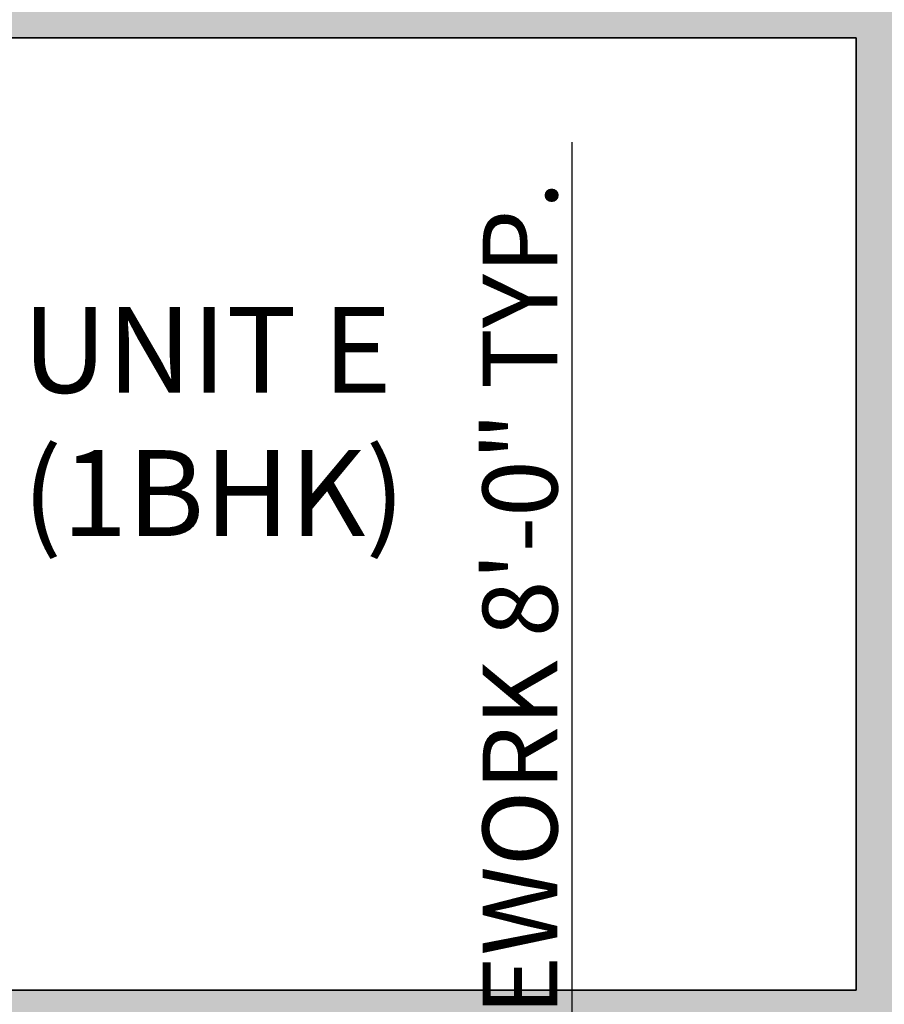
# Model space of a CAD drawing. Units: inches. Extents: x 2083 to 3317, y 1141 to 2115.
# Tile 89 of 256: x 2462 to 2600, y 1419 to 1577. Entities that reach past the tile are written whole.
import ezdxf

# ---------------------------------------------------------------- set-up
doc = ezdxf.new("R2010")
doc.units = ezdxf.units.IN
for name, color, linetype, lineweight in [('A-ANNO-DIMS', 2, 'Continuous', 18), ('A-AREA-IDEN', 7, 'Continuous', 25), ('A-WALL', 7, 'Continuous', 35)]:
    doc.layers.add(name, color=color, linetype=linetype, lineweight=lineweight)
doc.layers.add('A-WALL-PATT', color=251, linetype='Continuous', lineweight=13, true_color=0x636466)
doc.styles.get("Standard").update_dxf_attribs({"font": 'arial.ttf'})
doc.dimstyles.new('ISO-25', dxfattribs={"dimtxt": 12, "dimasz": 12, "dimexe": 1.25, "dimexo": 0.625, "dimtad": 1, "dimlunit": 3, "dimtxsty": 'Standard', "dimcen": 2.5, "dimadec": 0, "dimazin": 0, "dimtfac": 1, "dimtmove": 0, "dimatfit": 3, "dimfxl": 1, "dimarcsym": 0})

# ---------------------------------------------------------------- blocks, each defined once
blk = doc.blocks.new('*D24')
at = {"layer": 'A-ANNO-DIMS', "color": 0, "lineweight": -2, "transparency": 16777216}
for p, q in [((2550.36, 1368.26), (2550.36, 1556.98)), ((2536.58, 1368.26), (2551.61, 1368.26)), ((2550.36, 1284.26), (2550.36, 1356.26)), ((2536.58, 1272.26), (2551.61, 1272.26))]:
    blk.add_line(p, q, dxfattribs=at)
at = {"layer": 'A-ANNO-DIMS', "color": 0, "transparency": 16777216}
for points in [[(2548.36, 1356.26), (2552.36, 1356.26), (2550.36, 1368.26)], [(2548.36, 1284.26), (2552.36, 1284.26), (2550.36, 1272.26)]]:
    blk.add_solid(points, dxfattribs=at)
at = {"layer": 'Defpoints', "color": 0, "transparency": 16777216}
for p in [(2535.96, 1368.26), (2550.36, 1368.26), (2535.96, 1272.26)]:
    blk.add_point(p, dxfattribs=at)
at = {"layer": 'A-ANNO-DIMS', "color": 0, "transparency": 16777216, "insert": (2543.53, 1468.62), "char_height": 12, "attachment_point": 5, "rotation": 90}
blk.add_mtext('CASEWORK 8\'-0" TYP.', dxfattribs=at)

msp = doc.modelspace()

# ---------------------------------------------------------------- hatches: boundary and pattern name
at = {"layer": 'A-WALL-PATT'}
h = msp.add_hatch(color=256, dxfattribs=at)
h.dxf.hatch_style = 1
h.paths.add_polyline_path([(3126.96, 2020.761), (2748.96, 2020.761), (2604.96, 2020.761), (2226.96, 2020.761), (2226.96, 1702.761), (2466.96, 1702.761), (2466.96, 1582.761), (2418.96, 1582.761), (2418.96, 1477.761), (2226.96, 1477.761), (2226.96, 1263.261), (2544.96, 1263.261), (2544.96, 1411.761), (2604.96, 1411.761), (2685.96, 1411.761), (2685.96, 1420.761), (2604.96, 1420.761), (2604.96, 1573.761), (2604.96, 1702.761), (2604.96, 2011.761), (2748.96, 2011.761), (2748.96, 1702.761), (2862.96, 1702.761), (2862.96, 1621.761), (2871.96, 1621.761), (2871.96, 1702.761), (2883.96, 1702.761), (2883.96, 1706.939, -0.0264593), (2883.96, 1711.761), (2757.96, 1711.761), (2757.96, 1807.761), (2787.96, 1807.761), (2787.96, 1812.261), (2757.96, 1812.261), (2757.96, 2011.761), (2877.96, 2011.761), (2877.96, 1812.261), (2847.96, 1812.261), (2847.96, 1807.761), (2889.836, 1807.761), (2889.836, 1812.261), (2882.46, 1812.261), (2882.46, 2011.761), (3117.96, 2011.761), (3117.96, 1812.261), (2937.836, 1812.261), (2937.836, 1807.761), (2995.71, 1807.761), (2995.71, 1796.118), (3000.21, 1796.118), (3000.21, 1807.761), (3117.96, 1807.761), (3117.96, 1711.761), (3000.21, 1711.761), (3000.21, 1760.118), (2998.573, 1760.118, -0.020711), (2995.71, 1760.118), (2995.71, 1711.761), (2931.96, 1711.761), (2931.96, 1702.761), (3126.96, 1702.761)])
h.paths.add_polyline_path([(2471.46, 2011.761), (2471.46, 1810.011), (2462.717, 1810.011), (2462.717, 1805.511), (2505.96, 1805.511), (2505.96, 1810.011), (2475.96, 1810.011), (2475.96, 2011.761), (2595.96, 2011.761), (2595.96, 1810.011), (2565.96, 1810.011), (2565.96, 1805.511), (2595.96, 1805.511), (2595.96, 1711.761), (2235.96, 1711.761), (2235.96, 1805.511), (2353.71, 1805.511), (2353.71, 1796.054), (2358.21, 1796.054), (2358.21, 1805.511), (2414.717, 1805.511), (2414.717, 1810.011), (2235.96, 1810.011), (2235.96, 2011.761)], flags=16)
h.paths.add_polyline_path([(2270.205, 1994.61), (2270.205, 1970.61), (2246.205, 1970.61), (2246.205, 1994.61)], flags=0)
edge = h.paths.add_edge_path(flags=0)
edge.add_ellipse((2332.027, 1899.798), major_axis=(-3.043, 3.043), ratio=0.1682525, start_angle=-161.33217, end_angle=-156.30711, ccw=False)
edge.add_ellipse((2333.082, 1898.744), major_axis=(-1.055, 1.055), ratio=0.4535321, start_angle=-123.37102, end_angle=-94.15911)
edge = h.paths.add_edge_path(flags=0)
edge.add_ellipse((2332.027, 1968.876), major_axis=(3.043, 3.043), ratio=0.1682525, start_angle=18.66783, end_angle=23.69289)
edge.add_spline(control_points=[(2332.926, 1970.691), (2332.227, 1970.336), (2330.894, 1969.659), (2328.413, 1970.932), (2327.204, 1967.749), (2324.71, 1969.956), (2322.533, 1967.012), (2320.013, 1971.296), (2317.68, 1968.158), (2316.041, 1967.102), (2315.427, 1966.81)], knot_values=[0, 0, 0, 0, 2.2670587, 4.3245589, 6.6855835, 8.8786411, 11.121502, 14.300359, 17.7552837, 19.732645, 19.732645, 19.732645, 19.732645], degree=3, periodic=0)
edge.add_ellipse((2332.027, 1968.876), major_axis=(3.043, 3.043), ratio=0.1682525, start_angle=18.66783, end_angle=23.69289, ccw=False)
edge.add_ellipse((2333.082, 1969.931), major_axis=(1.055, 1.055), ratio=0.4535321, start_angle=56.62898, end_angle=85.84089, ccw=False)
edge = h.paths.add_edge_path(flags=0)
edge.add_spline(control_points=[(2296.428, 1967.988), (2293.628, 1965.336), (2287.704, 1959.727), (2299.744, 1949.996), (2294.533, 1935.669), (2290.573, 1920.604), (2293.394, 1909.974), (2296.185, 1904.967)], knot_values=[0.0991853, 0.0991853, 0.0991853, 0.0991853, 0.3453009, 0.6198217, 0.9826526, 1.3860932, 1.8105546, 1.8105546, 1.8105546, 1.8105546], degree=3, periodic=0)
edge.add_spline(control_points=[(2296.185, 1904.967), (2297.384, 1902.619), (2298.001, 1901.949), (2298.553, 1901.468)], knot_values=[0.0062457, 0.0062457, 0.0062457, 0.0062457, 0.0554759, 0.0554759, 0.0554759, 0.0554759], degree=3, periodic=0)
edge.add_spline(control_points=[(2298.553, 1901.468), (2297.259, 1900.923), (2295.225, 1900.232), (2293.06, 1900.614), (2292.101, 1900.788), (2292.09, 1900.791)], knot_values=[0.3128349, 0.3128349, 0.3128349, 0.3128349, 0.4017797, 0.4749867, 0.4759027, 0.4759027, 0.4759027, 0.4759027], degree=3, periodic=0)
edge.add_arc((2292.794, 1904.664), 3.937, 215.4209, 259.69818, ccw=False)
edge.add_spline(control_points=[(2289.585, 1902.382), (2289.477, 1902.535), (2289.368, 1902.688), (2289.261, 1902.841)], knot_values=[0.1028719, 0.1028719, 0.1028719, 0.1028719, 0.1168958, 0.1168958, 0.1168958, 0.1168958], degree=3, periodic=0)
edge.add_spline(control_points=[(2289.261, 1902.841), (2288.687, 1902.55), (2287.64, 1902.02), (2285.881, 1901.874), (2283.853, 1901.504), (2281.72, 1899.711), (2278.467, 1899.493), (2276.157, 1901.883), (2272.259, 1899.804), (2267.778, 1901.843), (2262.244, 1900.184), (2257.415, 1901.782), (2254.318, 1900.726), (2253.178, 1900.337)], knot_values=[0, 0, 0, 0, 1.9079767, 3.4771759, 5.261074, 7.9728515, 11.6802485, 13.7179214, 16.9395917, 22.789562, 27.5025027, 33.5952153, 37.1456181, 37.1456181, 37.1456181, 37.1456181], degree=3, periodic=0)
edge.add_line((2253.178, 1900.337), (2250.244, 1902.841))
edge.add_line((2250.244, 1902.841), (2250.244, 1965.833))
edge.add_line((2250.244, 1965.833), (2253.178, 1968.337))
edge.add_spline(control_points=[(2253.178, 1968.337), (2254.318, 1967.948), (2257.415, 1966.892), (2262.244, 1968.49), (2267.778, 1966.831), (2271.527, 1968.537), (2273.876, 1967.828), (2274.207, 1967.728)], knot_values=[0, 0, 0, 0, 0.0901802, 0.2449351, 0.3646438, 0.5132331, 0.5378548, 0.5378548, 0.5378548, 0.5378548], degree=3, periodic=0)
edge.add_arc((2274.353, 1963.793), 3.937, 72.05113, 92.12795, ccw=False)
edge.add_arc((2281.297, 1985.23), 18.596, 252.05113, 288.56572)
edge.add_arc((2292.317, 1956.029), 12.646, 71.02679, 113.77822, ccw=False)
edge = h.paths.add_edge_path(flags=0)
edge.add_spline(control_points=[(2274.899, 1951.856), (2275.066, 1951.617), (2275.233, 1951.377), (2275.398, 1951.136)], knot_values=[1.4099157, 1.4099157, 1.4099157, 1.4099157, 1.4315903, 1.4315903, 1.4315903, 1.4315903], degree=3, periodic=0)
edge.add_spline(control_points=[(2275.398, 1951.136), (2275.792, 1950.562), (2276.179, 1949.984), (2276.546, 1949.397)], knot_values=[1.3582378, 1.3582378, 1.3582378, 1.3582378, 1.4099157, 1.4099157, 1.4099157, 1.4099157], degree=3, periodic=0)
edge.add_line((2276.546, 1949.397), (2277.437, 1947.862))
edge.add_spline(control_points=[(2277.437, 1947.862), (2276.304, 1945.673), (2274.64, 1942.427), (2274.632, 1938.094), (2272.799, 1930.852), (2274.356, 1943.897), (2275.948, 1947.923), (2276.546, 1949.397)], knot_values=[0.0056315, 0.0056315, 0.0056315, 0.0056315, 0.1860139, 0.2660015, 0.3570872, 0.5963902, 0.7397317, 0.7397317, 0.7397317, 0.7397317], degree=3, periodic=0)
edge.add_spline(control_points=[(2276.546, 1949.397), (2276.179, 1949.984), (2275.792, 1950.562), (2275.398, 1951.136)], knot_values=[1.3582378, 1.3582378, 1.3582378, 1.3582378, 1.4099157, 1.4099157, 1.4099157, 1.4099157], degree=3, periodic=0)
edge.add_spline(control_points=[(2275.398, 1951.136), (2274.943, 1950.08), (2274.208, 1948.025), (2273.935, 1944.851), (2272.469, 1937.627), (2273.466, 1945.696), (2274.701, 1951.059), (2274.899, 1951.856)], knot_values=[0.1043639, 0.1043639, 0.1043639, 0.1043639, 0.1896363, 0.2696239, 0.3607096, 0.6000126, 0.6446217, 0.6446217, 0.6446217, 0.6446217], degree=3, periodic=0)
h.paths.add_polyline_path([(2269.168, 1963.128, -0.3575267), (2268.171, 1960.976, -0.0925607), (2268.171, 1939.436, -0.3575267), (2269.168, 1937.285, -0.3575267), (2267.016, 1938.282, -0.1647847), (2254.686, 1938.282, -0.3575267), (2252.534, 1937.285, -0.3575267), (2253.531, 1939.436, -0.0925607), (2253.531, 1960.976, -0.3575267), (2252.534, 1963.128, -0.3575267), (2254.686, 1962.131, -0.1647847), (2267.016, 1962.131, -0.3575267)], flags=0)
h.paths.add_polyline_path([(2248.874, 1967.802), (2248.874, 1957.028), (2249.458, 1957.028), (2249.458, 1911.647), (2248.874, 1911.647), (2248.874, 1900.873), (2246.512, 1900.873, 0.1973271), (2244.15, 1902.457), (2244.15, 1966.218, 0.1973271), (2246.512, 1967.802)], flags=0)
h.paths.add_polyline_path([(2269.168, 1931.389, -0.3575267), (2268.171, 1929.238, -0.0925607), (2268.171, 1907.698, -0.3575267), (2269.168, 1905.547, -0.3575267), (2267.016, 1906.544, -0.1647847), (2254.686, 1906.544, -0.3575267), (2252.534, 1905.547, -0.3575267), (2253.531, 1907.698, -0.0925607), (2253.531, 1929.238, -0.3575267), (2252.534, 1931.389, -0.3575267), (2254.686, 1930.392, -0.1647847), (2267.016, 1930.392, -0.3575267)], flags=0)
edge = h.paths.add_edge_path(flags=0)
edge.add_spline(control_points=[(2276.197, 1906.724), (2276.168, 1909.029), (2276.114, 1913.372), (2270.598, 1924.925), (2273.905, 1919.013), (2275.922, 1916.262), (2275.475, 1912.402), (2277.258, 1910.381), (2276.696, 1908.225), (2276.646, 1906.813), (2276.618, 1906.008)], knot_values=[0, 0, 0, 0, 8.6102597, 16.2212739, 18.8430575, 23.8048978, 27.4408283, 29.3561016, 31.2034776, 33.6506866, 33.6506866, 33.6506866, 33.6506866], degree=3, periodic=0)
edge.add_spline(control_points=[(2276.618, 1906.008), (2276.623, 1905.624), (2276.498, 1904.629), (2275.442, 1903.855), (2274.937, 1903.08), (2274.859, 1902.841)], knot_values=[0.1564884, 0.1564884, 0.1564884, 0.1564884, 0.1843975, 0.2313765, 0.2505985, 0.2505985, 0.2505985, 0.2505985], degree=3, periodic=0)
edge.add_line((2274.859, 1902.841), (2276.506, 1902.841))
edge.add_spline(control_points=[(2276.506, 1902.841), (2276.788, 1903.085), (2277.665, 1904.125), (2278.25, 1904.341), (2277.654, 1908.527), (2278.156, 1906.228), (2278.1, 1905.286), (2278.847, 1904.069), (2277.857, 1903.415), (2277.874, 1902.991), (2277.904, 1902.841)], knot_values=[0.0595743, 0.0595743, 0.0595743, 0.0595743, 0.0807529, 0.1037415, 0.1697201, 0.1760361, 0.2071372, 0.2404744, 0.2623409, 0.2736605, 0.2736605, 0.2736605, 0.2736605], degree=3, periodic=0)
edge.add_line((2277.904, 1902.841), (2280.03, 1902.841))
edge.add_spline(control_points=[(2280.03, 1902.841), (2279.888, 1903.088), (2279.499, 1903.982), (2280.152, 1905.939), (2278.104, 1909.658), (2279.762, 1907.185), (2280.328, 1904.875), (2280.485, 1903.49), (2281.463, 1903.249), (2281.758, 1902.936), (2281.834, 1902.841)], knot_values=[0.013856, 0.013856, 0.013856, 0.013856, 0.0348738, 0.0888667, 0.1078792, 0.1267378, 0.158714, 0.1937575, 0.2174868, 0.2267221, 0.2267221, 0.2267221, 0.2267221], degree=3, periodic=0)
edge.add_spline(control_points=[(2281.834, 1902.841), (2281.788, 1902.827), (2281.647, 1902.783), (2281.396, 1902.859), (2281.088, 1902.985), (2280.721, 1903.061), (2280.333, 1903.026), (2280.125, 1902.899), (2280.03, 1902.841)], knot_values=[0, 0, 0, 0, 0.1441304, 0.435517, 0.7492759, 1.1530457, 1.5483707, 1.878348, 1.878348, 1.878348, 1.878348], degree=3, periodic=0)
edge.add_line((2280.03, 1902.841), (2277.904, 1902.841))
edge.add_spline(control_points=[(2277.904, 1902.841), (2277.893, 1902.796), (2277.865, 1902.68), (2277.607, 1902.687), (2277.274, 1902.801), (2276.838, 1902.62), (2276.584, 1902.789), (2276.506, 1902.841)], knot_values=[0, 0, 0, 0, 0.1271885, 0.3261988, 0.6280094, 1.2435704, 1.5153306, 1.5153306, 1.5153306, 1.5153306], degree=3, periodic=0)
edge.add_line((2276.506, 1902.841), (2274.859, 1902.841))
edge.add_spline(control_points=[(2274.859, 1902.841), (2274.814, 1902.899), (2274.725, 1903.013), (2274.493, 1903.119), (2274.244, 1902.961), (2273.937, 1903.185), (2273.614, 1902.983), (2273.408, 1902.883), (2273.322, 1902.841)], knot_values=[0, 0, 0, 0, 0.2184302, 0.4369566, 0.6879766, 0.9903786, 1.3983955, 1.6918498, 1.6918498, 1.6918498, 1.6918498], degree=3, periodic=0)
edge.add_spline(control_points=[(2273.322, 1902.841), (2273.617, 1903.446), (2274.274, 1904.538), (2276.027, 1904.574), (2276.207, 1906.584), (2276.197, 1906.724)], knot_values=[0.0122268, 0.0122268, 0.0122268, 0.0122268, 0.0594721, 0.1062177, 0.134458, 0.134458, 0.134458, 0.134458], degree=3, periodic=0)
h.paths.add_polyline_path([(2270.776, 1897.79), (2270.776, 1873.79), (2246.776, 1873.79), (2246.776, 1897.79)], flags=0)
h.paths.add_polyline_path([(2353.71, 1760.005), (2353.71, 1760.054), (2358.21, 1760.054, -0.033729)], flags=0)
h.paths.add_polyline_path([(2321.819, 1737.529), (2341.995, 1737.529, -0.4142136), (2343.203, 1736.321), (2343.203, 1721.021, -0.4142136), (2341.995, 1719.813), (2321.819, 1719.813, -0.4142136), (2320.611, 1721.021), (2320.611, 1736.321, -0.4142136)], flags=0)
h.paths.add_polyline_path([(2324.235, 1736.321), (2339.579, 1736.321, -0.4142136), (2341.995, 1733.905), (2341.995, 1725.45, -0.4142136), (2339.579, 1723.034), (2333.681, 1723.034), (2333.845, 1722.045, -0.8706461), (2335.425, 1721.826, -0.767327), (2333.923, 1721.423), (2331.291, 1721.423, -0.767327), (2329.788, 1721.826, -0.8706461), (2331.368, 1722.045), (2331.533, 1723.034), (2324.235, 1723.034, -0.4142136), (2321.819, 1725.45), (2321.819, 1733.905, -0.4142136)], flags=0)
h.paths.add_polyline_path([(2570.484, 1928.615), (2589.684, 1928.615), (2590.169, 1928.615), (2590.169, 1904.993), (2570.484, 1904.993)], flags=0)
h.paths.add_polyline_path([(2574.447, 1927.264, -1), (2572.829, 1927.264, -1)], flags=0)
h.paths.add_polyline_path([(2573.09, 1926.941), (2573.925, 1927.776), (2574.148, 1927.553), (2573.313, 1926.718)], flags=0)
h.paths.add_polyline_path([(2578.779, 1919.73, -1), (2571.592, 1919.73, -1)], flags=0)
h.paths.add_polyline_path([(2578.385, 1919.73, -1), (2571.985, 1919.73, -1)], flags=0)
h.paths.add_polyline_path([(2331.596, 1729.476, -1), (2333.618, 1729.476, -1)], flags=0)
h.paths.add_polyline_path([(2578.034, 1927.264, -1), (2576.416, 1927.264, -1)], flags=0)
h.paths.add_polyline_path([(2576.689, 1927.531), (2576.912, 1927.754), (2577.747, 1926.919), (2577.524, 1926.696)], flags=0)
h.paths.add_polyline_path([(2578.139, 1909.86, -1), (2572.232, 1909.86, -1)], flags=0)
h.paths.add_polyline_path([(2577.745, 1909.86, -1), (2572.625, 1909.86, -1)], flags=0)
h.paths.add_polyline_path([(2583.798, 1927.264, -1), (2582.179, 1927.264, -1)], flags=0)
h.paths.add_polyline_path([(2582.719, 1927.754), (2583.554, 1926.919), (2583.331, 1926.696), (2582.496, 1927.531)], flags=0)
h.paths.add_polyline_path([(2582.496, 1927.531), (2582.719, 1927.754), (2583.554, 1926.919), (2583.331, 1926.696)], flags=0)
h.paths.add_polyline_path([(2587.739, 1920.53, -1), (2581.832, 1920.53, -1)], flags=0)
h.paths.add_polyline_path([(2587.345, 1920.53, -1), (2582.225, 1920.53, -1)], flags=0)
h.paths.add_polyline_path([(2587.385, 1927.264, -1), (2585.766, 1927.264, -1)], flags=0)
h.paths.add_polyline_path([(2586.082, 1926.98), (2586.917, 1927.815), (2587.14, 1927.593), (2586.305, 1926.758)], flags=0)
h.paths.add_polyline_path([(2588.379, 1910.66, -1), (2581.192, 1910.66, -1)], flags=0)
h.paths.add_polyline_path([(2587.985, 1910.66, -1), (2581.585, 1910.66, -1)], flags=0)
h.paths.add_polyline_path([(2417.168, 1729.478), (2437.344, 1729.478, -0.4142136), (2438.552, 1728.27), (2438.552, 1712.969, -0.4142136), (2437.344, 1711.761), (2417.168, 1711.761, -0.4142136), (2415.96, 1712.969), (2415.96, 1728.27, -0.4142136)], flags=0)
h.paths.add_polyline_path([(2419.584, 1728.27), (2434.928, 1728.27, -0.4142136), (2437.344, 1725.854), (2437.344, 1717.398, -0.4142136), (2434.928, 1714.983), (2429.029, 1714.983), (2429.194, 1713.994, -0.8706461), (2430.774, 1713.775, -0.767327), (2429.271, 1713.372), (2426.64, 1713.372, -0.767327), (2425.137, 1713.775, -0.8706461), (2426.717, 1713.994), (2426.882, 1714.983), (2419.584, 1714.983, -0.4142136), (2417.168, 1717.398), (2417.168, 1725.854, -0.4142136)], flags=0)
h.paths.add_polyline_path([(2419.584, 1728.27), (2434.928, 1728.27, -0.4142136), (2437.344, 1725.854), (2437.344, 1717.398, -0.4142136), (2434.928, 1714.983), (2429.029, 1714.983), (2428.358, 1719.009), (2427.553, 1719.009), (2426.882, 1714.983), (2419.584, 1714.983, -0.4142136), (2417.168, 1717.398), (2417.168, 1725.854, -0.4142136)], flags=0)
h.paths.add_polyline_path([(2426.944, 1721.425, -1), (2428.967, 1721.425, -1)], flags=0)
h.paths.add_polyline_path([(2475.96, 1702.761), (2595.96, 1702.761), (2595.96, 1582.761), (2475.96, 1582.761)], flags=16)
h.paths.add_polyline_path([(2427.96, 1573.761), (2595.96, 1573.761), (2595.96, 1468.761), (2595.96, 1420.761), (2384.46, 1420.761), (2384.46, 1468.761), (2427.96, 1468.761)], flags=16)
h.paths.add_polyline_path([(2379.96, 1468.761), (2379.96, 1420.761), (2235.96, 1420.761), (2235.96, 1468.761)], flags=16)
h.paths.add_polyline_path([(2317.816, 1466.696), (2337.992, 1466.696, -0.4142136), (2339.2, 1465.488), (2339.2, 1450.187, -0.4142136), (2337.992, 1448.979), (2317.816, 1448.979, -0.4142136), (2316.608, 1450.187), (2316.608, 1465.488, -0.4142136)], flags=0)
h.paths.add_polyline_path([(2320.232, 1465.488), (2335.576, 1465.488, -0.4142136), (2337.992, 1463.072), (2337.992, 1454.616, -0.4142136), (2335.576, 1452.2), (2329.677, 1452.2), (2329.842, 1451.212, -0.8706461), (2331.422, 1450.992, -0.767327), (2329.92, 1450.59), (2327.288, 1450.59, -0.767327), (2325.785, 1450.992, -0.8706461), (2327.365, 1451.212), (2327.53, 1452.2), (2320.232, 1452.2, -0.4142136), (2317.816, 1454.616), (2317.816, 1463.072, -0.4142136)], flags=0)
h.paths.add_polyline_path([(2320.232, 1465.488), (2335.576, 1465.488, -0.4142136), (2337.992, 1463.072), (2337.992, 1454.616, -0.4142136), (2335.576, 1452.2), (2329.677, 1452.2), (2329.006, 1456.227), (2328.201, 1456.227), (2327.53, 1452.2), (2320.232, 1452.2, -0.4142136), (2317.816, 1454.616), (2317.816, 1463.072, -0.4142136)], flags=0)
h.paths.add_polyline_path([(2327.593, 1458.643, -1), (2329.615, 1458.643, -1)], flags=0)
h.paths.add_polyline_path([(2244.412, 1433.34), (2241.921, 1433.34, -0.4142136), (2240.018, 1435.244), (2240.018, 1440.953, -0.4142105), (2241.921, 1442.856), (2244.412, 1442.856, -1.9764724)], flags=0)
h.paths.add_polyline_path([(2245.357, 1434.398, -0.4142136), (2245.357, 1441.799, -2.1440985)], flags=0)
h.paths.add_polyline_path([(2535.96, 1416.261), (2535.96, 1272.261), (2235.96, 1272.261), (2235.96, 1416.261)], flags=16)
h.paths.add_polyline_path([(2260.12, 1384.293), (2260.12, 1362.039), (2237.865, 1362.039), (2237.865, 1384.293)], flags=0)
edge = h.paths.add_edge_path(flags=0)
edge.add_line((2318.252, 1362.093), (2318.146, 1362.001))
edge.add_ellipse((2317.445, 1360.431), major_axis=(2.822, 2.822), ratio=0.1682525, start_angle=18.66783, end_angle=20.94813, ccw=False)
edge.add_ellipse((2318.423, 1361.409), major_axis=(0.978, 0.978), ratio=0.4535321, start_angle=56.62898, end_angle=70.2262, ccw=False)
edge = h.paths.add_edge_path(flags=0)
edge.add_line((2319.107, 1295.571), (2319.015, 1295.677))
edge.add_ellipse((2317.445, 1296.378), major_axis=(-2.822, 2.822), ratio=0.1682525, start_angle=-161.33217, end_angle=-159.05187, ccw=False)
edge.add_ellipse((2318.423, 1295.4), major_axis=(-0.978, 0.978), ratio=0.4535321, start_angle=-123.37102, end_angle=-109.7738)
edge = h.paths.add_edge_path(flags=0)
edge.add_spline(control_points=[(2284.21, 1301.17), (2284.581, 1300.445), (2284.891, 1299.892), (2285.16, 1299.461)], knot_values=[0.0390658, 0.0390658, 0.0390658, 0.0390658, 0.0554759, 0.0554759, 0.0554759, 0.0554759], degree=3, periodic=0)
edge.add_line((2285.16, 1299.461), (2284.21, 1301.17))
edge = h.paths.add_edge_path(flags=0)
edge.add_line((2280.412, 1297.298), (2283.37, 1297.036))
edge.add_line((2283.37, 1297.036), (2286.406, 1297.926))
edge.add_spline(control_points=[(2286.406, 1297.926), (2285.305, 1297.463), (2284.345, 1297.129), (2283.37, 1297.036)], knot_values=[0.3943688, 0.3943688, 0.3943688, 0.3943688, 0.4759027, 0.4759027, 0.4759027, 0.4759027], degree=3, periodic=0)
edge.add_spline(control_points=[(2283.37, 1297.036), (2283.281, 1297.028), (2282.316, 1296.957), (2281.313, 1297.134), (2280.423, 1297.296), (2280.412, 1297.298)], knot_values=[0.3128349, 0.3128349, 0.3128349, 0.3128349, 0.3202458, 0.3934528, 0.3943688, 0.3943688, 0.3943688, 0.3943688], degree=3, periodic=0)
edge = h.paths.add_edge_path(flags=0)
edge.add_line((2284.436, 1359.607), (2280.446, 1355.328))
edge.add_line((2280.446, 1355.328), (2279.58, 1351.018))
edge.add_line((2279.58, 1351.018), (2282.413, 1346.58))
edge.add_spline(control_points=[(2282.413, 1346.58), (2283.153, 1345.589), (2284.253, 1344.029), (2284.801, 1342.387), (2284.935, 1341.806)], knot_values=[1.2400982, 1.2400982, 1.2400982, 1.2400982, 1.3328922, 1.3827123, 1.3827123, 1.3827123, 1.3827123], degree=3, periodic=0)
edge.add_spline(control_points=[(2284.935, 1341.806), (2285.319, 1340.141), (2285.233, 1338.409), (2284.91, 1336.654)], knot_values=[1.0974841, 1.0974841, 1.0974841, 1.0974841, 1.2400982, 1.2400982, 1.2400982, 1.2400982], degree=3, periodic=0)
edge.add_spline(control_points=[(2284.91, 1336.654), (2284.587, 1334.899), (2284.027, 1333.12), (2283.463, 1331.361)], knot_values=[0.9548699, 0.9548699, 0.9548699, 0.9548699, 1.0974841, 1.0974841, 1.0974841, 1.0974841], degree=3, periodic=0)
edge.add_line((2283.463, 1331.361), (2281.89, 1326.153))
edge.add_line((2281.89, 1326.153), (2280.756, 1321.056))
edge.add_line((2280.756, 1321.056), (2280.299, 1316.002))
edge.add_line((2280.299, 1316.002), (2280.716, 1310.95))
edge.add_line((2280.716, 1310.95), (2282.028, 1305.972))
edge.add_line((2282.028, 1305.972), (2284.21, 1301.17))
edge.add_spline(control_points=[(2284.21, 1301.17), (2283.341, 1302.73), (2282.612, 1304.336), (2282.028, 1305.972)], knot_values=[0.0991853, 0.0991853, 0.0991853, 0.0991853, 0.2417994, 0.2417994, 0.2417994, 0.2417994], degree=3, periodic=0)
edge.add_spline(control_points=[(2282.028, 1305.972), (2281.444, 1307.608), (2281.005, 1309.273), (2280.716, 1310.95)], knot_values=[0.2417994, 0.2417994, 0.2417994, 0.2417994, 0.3844135, 0.3844135, 0.3844135, 0.3844135], degree=3, periodic=0)
edge.add_spline(control_points=[(2280.716, 1310.95), (2280.433, 1312.588), (2280.289, 1314.277), (2280.299, 1315.962), (2280.299, 1316.002)], knot_values=[0.3844135, 0.3844135, 0.3844135, 0.3844135, 0.5236467, 0.5270276, 0.5270276, 0.5270276, 0.5270276], degree=3, periodic=0)
edge.add_spline(control_points=[(2280.299, 1316.002), (2280.312, 1317.687), (2280.478, 1319.368), (2280.756, 1321.056)], knot_values=[0.5270276, 0.5270276, 0.5270276, 0.5270276, 0.6696417, 0.6696417, 0.6696417, 0.6696417], degree=3, periodic=0)
edge.add_spline(control_points=[(2280.756, 1321.056), (2281.035, 1322.744), (2281.426, 1324.44), (2281.89, 1326.153)], knot_values=[0.6696417, 0.6696417, 0.6696417, 0.6696417, 0.8122558, 0.8122558, 0.8122558, 0.8122558], degree=3, periodic=0)
edge.add_spline(control_points=[(2281.89, 1326.153), (2282.264, 1327.533), (2282.788, 1329.262), (2283.353, 1331.018), (2283.463, 1331.361)], knot_values=[0.8122558, 0.8122558, 0.8122558, 0.8122558, 0.9270873, 0.9548699, 0.9548699, 0.9548699, 0.9548699], degree=3, periodic=0)
edge.add_line((2283.463, 1331.361), (2284.91, 1336.654))
edge.add_line((2284.91, 1336.654), (2284.935, 1341.806))
edge.add_line((2284.935, 1341.806), (2282.413, 1346.58))
edge.add_spline(control_points=[(2282.413, 1346.58), (2281.275, 1348.104), (2280.078, 1349.57), (2279.58, 1351.018)], knot_values=[1.3827123, 1.3827123, 1.3827123, 1.3827123, 1.5253264, 1.5253264, 1.5253264, 1.5253264], degree=3, periodic=0)
edge.add_spline(control_points=[(2279.58, 1351.018), (2279.443, 1351.415), (2279.136, 1352.857), (2279.735, 1354.29), (2280.446, 1355.328)], knot_values=[1.5253264, 1.5253264, 1.5253264, 1.5253264, 1.564439, 1.6679405, 1.6679405, 1.6679405, 1.6679405], degree=3, periodic=0)
edge.add_spline(control_points=[(2280.446, 1355.328), (2281.426, 1356.758), (2282.931, 1358.183), (2284.436, 1359.607)], knot_values=[1.6679405, 1.6679405, 1.6679405, 1.6679405, 1.8105546, 1.8105546, 1.8105546, 1.8105546], degree=3, periodic=0)
edge.add_arc((2280.623, 1348.518), 11.726, 71.02679, 113.77822)
edge.add_arc((2270.405, 1375.595), 17.244, 252.05113, 288.56572, ccw=False)
edge.add_arc((2263.966, 1355.718), 3.651, 72.05113, 92.12795)
edge.add_arc((2263.966, 1355.718), 3.651, 92.12795, 177.98513)
edge.add_spline(control_points=[(2260.318, 1355.846), (2260.26, 1354.221), (2260.551, 1350.187), (2262.999, 1346.766), (2264.473, 1344.649)], knot_values=[1.4315903, 1.4315903, 1.4315903, 1.4315903, 1.5641438, 1.7706953, 1.7706953, 1.7706953, 1.7706953], degree=3, periodic=0)
edge.add_line((2264.473, 1344.649), (2264.936, 1343.983))
edge.add_spline(control_points=[(2263.801, 1340.248), (2263.843, 1340.514), (2264.067, 1341.756), (2264.513, 1343.002), (2264.935, 1343.981)], knot_values=[0.5365702, 0.5365702, 0.5365702, 0.5365702, 0.5593494, 0.6446217, 0.6446217, 0.6446217, 0.6446217], degree=3, periodic=0)
edge.add_spline(control_points=[(2264.935, 1343.981), (2265.118, 1343.715), (2265.299, 1343.448), (2265.477, 1343.179)], knot_values=[1.3840767, 1.3840767, 1.3840767, 1.3840767, 1.4099157, 1.4099157, 1.4099157, 1.4099157], degree=3, periodic=0)
edge.add_spline(control_points=[(2265.477, 1343.179), (2265.655, 1342.911), (2265.829, 1342.641), (2265.999, 1342.369)], knot_values=[1.3582378, 1.3582378, 1.3582378, 1.3582378, 1.3840767, 1.3840767, 1.3840767, 1.3840767], degree=3, periodic=0)
edge.add_line((2265.999, 1342.369), (2266.826, 1340.946))
edge.add_spline(control_points=[(2266.826, 1340.946), (2268.894, 1337.09), (2271.398, 1325.843), (2270.516, 1310.569), (2275.919, 1301.861), (2277.79, 1299.199)], knot_values=[0.1168958, 0.1168958, 0.1168958, 0.1168958, 0.4729873, 1.0509689, 1.3137934, 1.3137934, 1.3137934, 1.3137934], degree=3, periodic=0)
edge.add_spline(control_points=[(2277.79, 1299.199), (2277.839, 1299.128), (2277.889, 1299.057), (2277.94, 1298.987)], knot_values=[0.1098839, 0.1098839, 0.1098839, 0.1098839, 0.1168958, 0.1168958, 0.1168958, 0.1168958], degree=3, periodic=0)
edge.add_line((2277.94, 1298.987), (2277.789, 1299.199))
edge.add_spline(control_points=[(2277.789, 1299.199), (2277.257, 1298.929), (2276.286, 1298.438), (2275.039, 1298.334), (2274.383, 1298.239), (2274.215, 1298.209)], knot_values=[33.1218702, 33.1218702, 33.1218702, 33.1218702, 35.0290557, 36.5982549, 37.1448269, 37.1448269, 37.1448269, 37.1448269], degree=3, periodic=0)
edge.add_line((2274.215, 1298.209), (2273.073, 1297.893))
edge.add_spline(control_points=[(2273.073, 1297.893), (2272.323, 1297.58), (2271.039, 1296.511), (2269.248, 1296.226), (2268.423, 1296.375)], knot_values=[26.5325843, 26.5325843, 26.5325843, 26.5325843, 29.198919, 31.8391012, 31.8391012, 31.8391012, 31.8391012], degree=3, periodic=0)
edge.add_line((2268.423, 1296.375), (2263.879, 1297.458))
edge.add_spline(control_points=[(2263.879, 1297.458), (2263.556, 1297.359), (2261.86, 1296.839), (2260.239, 1297.282), (2258.933, 1297.516)], knot_values=[15.9195506, 15.9195506, 15.9195506, 15.9195506, 16.9395917, 21.2260675, 21.2260675, 21.2260675, 21.2260675], degree=3, periodic=0)
edge.add_line((2258.933, 1297.516), (2254.055, 1297.329))
edge.add_spline(control_points=[(2254.055, 1297.329), (2253.756, 1297.296), (2252.114, 1297.165), (2250.462, 1297.544), (2249.13, 1297.668)], knot_values=[5.3065169, 5.3065169, 5.3065169, 5.3065169, 6.2764352, 10.6130337, 10.6130337, 10.6130337, 10.6130337], degree=3, periodic=0)
edge.add_line((2249.13, 1297.668), (2244.332, 1296.878))
edge.add_line((2244.332, 1296.878), (2241.611, 1299.199))
edge.add_line((2241.611, 1299.199), (2241.611, 1357.609))
edge.add_line((2241.611, 1357.609), (2244.332, 1359.931))
edge.add_line((2244.332, 1359.931), (2252.729, 1359.543))
edge.add_spline(control_points=[(2252.729, 1359.543), (2252.871, 1359.546), (2253.306, 1359.548), (2253.74, 1359.514), (2254.032, 1359.482)], knot_values=[0.233291, 0.233291, 0.233291, 0.233291, 0.2449351, 0.2689274, 0.2689274, 0.2689274, 0.2689274], degree=3, periodic=0)
edge.add_line((2254.032, 1359.482), (2259.587, 1359.416))
edge.add_spline(control_points=[(2259.587, 1359.416), (2260.677, 1359.629), (2262.073, 1359.897), (2263.524, 1359.459), (2263.83, 1359.366)], knot_values=[0.4225164, 0.4225164, 0.4225164, 0.4225164, 0.5132331, 0.5378548, 0.5378548, 0.5378548, 0.5378548], degree=3, periodic=0)
edge.add_arc((2263.966, 1355.718), 3.651, 72.05113, 92.12795, ccw=False)
edge.add_arc((2270.405, 1375.595), 17.244, 252.05113, 288.56572)
edge.add_arc((2280.623, 1348.518), 11.726, 71.02679, 113.77822, ccw=False)
h.paths.add_polyline_path([(2240.341, 1359.435), (2240.341, 1349.444), (2240.882, 1349.444), (2240.882, 1307.365), (2240.341, 1307.365), (2240.341, 1297.374), (2238.15, 1297.374, 0.1973271), (2235.96, 1298.843), (2235.96, 1357.966, 0.1973271), (2238.15, 1359.435)], flags=0)
h.paths.add_polyline_path([(2259.158, 1355.101, -0.3575267), (2258.233, 1353.106, -0.0925607), (2258.233, 1333.133, -0.3575267), (2259.158, 1331.138, -0.3575267), (2257.163, 1332.062, -0.1647847), (2245.729, 1332.062, -0.3575267), (2243.735, 1331.138, -0.3575267), (2244.659, 1333.133, -0.0925607), (2244.659, 1353.106, -0.3575267), (2243.735, 1355.101, -0.3575267), (2245.729, 1354.176, -0.1647847), (2257.163, 1354.176, -0.3575267)], flags=0)
edge = h.paths.add_edge_path(flags=0)
edge.add_line((2265.999, 1342.369), (2266.826, 1340.946))
edge.add_line((2266.826, 1340.946), (2265.308, 1337.814))
edge.add_line((2265.308, 1337.814), (2264.358, 1334.653))
edge.add_line((2264.358, 1334.653), (2264.262, 1333.8))
edge.add_spline(control_points=[(2264.262, 1333.8), (2264.208, 1333.187), (2264.162, 1332.366), (2264.007, 1331.414), (2263.969, 1331.202)], knot_values=[0.4644442, 0.4644442, 0.4644442, 0.4644442, 0.5166905, 0.5316081, 0.5316081, 0.5316081, 0.5316081], degree=3, periodic=0)
edge.add_spline(control_points=[(2263.969, 1331.202), (2263.775, 1330.119), (2263.424, 1328.791), (2263.257, 1328.531), (2263.234, 1328.515)], knot_values=[0.3726816, 0.3726816, 0.3726816, 0.3726816, 0.4488497, 0.4644442, 0.4644442, 0.4644442, 0.4644442], degree=3, periodic=0)
edge.add_spline(control_points=[(2263.234, 1328.515), (2263.096, 1328.42), (2263.131, 1329.301), (2263.275, 1330.616)], knot_values=[0.2809191, 0.2809191, 0.2809191, 0.2809191, 0.3726816, 0.3726816, 0.3726816, 0.3726816], degree=3, periodic=0)
edge.add_spline(control_points=[(2263.275, 1330.616), (2263.419, 1331.93), (2263.672, 1333.677), (2263.97, 1335.315)], knot_values=[0.1891566, 0.1891566, 0.1891566, 0.1891566, 0.2809191, 0.2809191, 0.2809191, 0.2809191], degree=3, periodic=0)
edge.add_spline(control_points=[(2263.97, 1335.315), (2264.1, 1336.032), (2264.419, 1337.622), (2264.755, 1338.864), (2264.947, 1339.491)], knot_values=[0.097394, 0.097394, 0.097394, 0.097394, 0.1375775, 0.1891566, 0.1891566, 0.1891566, 0.1891566], degree=3, periodic=0)
edge.add_spline(control_points=[(2264.947, 1339.491), (2265.29, 1340.606), (2265.644, 1341.494), (2265.999, 1342.369)], knot_values=[0.0056315, 0.0056315, 0.0056315, 0.0056315, 0.097394, 0.097394, 0.097394, 0.097394], degree=3, periodic=0)
h.paths.add_polyline_path([(2259.158, 1325.671, -0.3575267), (2258.233, 1323.676, -0.0925607), (2258.233, 1303.703, -0.3575267), (2259.158, 1301.708, -0.3575267), (2257.163, 1302.633, -0.1647847), (2245.729, 1302.633, -0.3575267), (2243.735, 1301.708, -0.3575267), (2244.659, 1303.703, -0.0925607), (2244.659, 1323.676, -0.3575267), (2243.735, 1325.671, -0.3575267), (2245.729, 1324.747, -0.1647847), (2257.163, 1324.747, -0.3575267)], flags=0)
edge = h.paths.add_edge_path(flags=0)
edge.add_spline(control_points=[(2261.709, 1317.311), (2261.679, 1317.418), (2261.762, 1317.389), (2262.491, 1316.09), (2262.962, 1315.301)], knot_values=[14.9558607, 14.9558607, 14.9558607, 14.9558607, 16.2212739, 18.6948259, 18.6948259, 18.6948259, 18.6948259], degree=3, periodic=0)
edge.add_spline(control_points=[(2262.962, 1315.301), (2262.99, 1315.254), (2263.702, 1314.067), (2264.349, 1313.127), (2264.73, 1312.164)], knot_values=[18.6948259, 18.6948259, 18.6948259, 18.6948259, 18.8430575, 22.433791, 22.433791, 22.433791, 22.433791], degree=3, periodic=0)
edge.add_spline(control_points=[(2264.73, 1312.164), (2264.876, 1311.796), (2265.177, 1310.77), (2265.143, 1309.559), (2265.248, 1308.824)], knot_values=[22.433791, 22.433791, 22.433791, 22.433791, 23.8048978, 26.1727562, 26.1727562, 26.1727562, 26.1727562], degree=3, periodic=0)
edge.add_line((2265.248, 1308.824), (2265.851, 1307.172))
edge.add_spline(control_points=[(2265.851, 1307.172), (2266.065, 1306.822), (2266.384, 1306.332), (2266.424, 1305.781), (2266.42, 1305.611)], knot_values=[28.0625624, 28.0625624, 28.0625624, 28.0625624, 29.3561016, 29.9117214, 29.9117214, 29.9117214, 29.9117214], degree=3, periodic=0)
edge.add_spline(control_points=[(2266.42, 1305.611), (2266.416, 1305.433), (2266.394, 1305.25), (2266.365, 1305.066)], knot_values=[29.9117214, 29.9117214, 29.9117214, 29.9117214, 30.4978371, 30.4978371, 30.4978371, 30.4978371], degree=3, periodic=0)
edge.add_line((2266.365, 1305.066), (2266.066, 1302.136))
edge.add_spline(control_points=[(2266.066, 1302.136), (2266.071, 1301.78), (2265.998, 1301.2), (2265.663, 1300.759), (2265.509, 1300.586)], knot_values=[0.1564884, 0.1564884, 0.1564884, 0.1564884, 0.1843975, 0.2035434, 0.2035434, 0.2035434, 0.2035434], degree=3, periodic=0)
edge.add_line((2265.509, 1300.586), (2264.435, 1299.199))
edge.add_line((2264.435, 1299.199), (2265.962, 1299.199))
edge.add_line((2265.962, 1299.199), (2267.336, 1301.175))
edge.add_line((2267.336, 1301.175), (2267.312, 1301.986))
edge.add_spline(control_points=[(2267.312, 1301.986), (2267.261, 1302.862), (2267.16, 1303.737), (2267.271, 1303.326)], knot_values=[0.1262286, 0.1262286, 0.1262286, 0.1262286, 0.1666174, 0.1666174, 0.1666174, 0.1666174], degree=3, periodic=0)
edge.add_spline(control_points=[(2267.271, 1303.326), (2267.28, 1303.294), (2267.31, 1303.175), (2267.373, 1302.884), (2267.406, 1302.683), (2267.418, 1302.601)], knot_values=[0.1666174, 0.1666174, 0.1666174, 0.1666174, 0.1697201, 0.1760361, 0.1807647, 0.1807647, 0.1807647, 0.1807647], degree=3, periodic=0)
edge.add_spline(control_points=[(2267.744, 1300.988), (2267.688, 1301.151), (2267.481, 1301.657), (2267.484, 1302.145), (2267.418, 1302.601)], knot_values=[0.1807647, 0.1807647, 0.1807647, 0.1807647, 0.1937665, 0.2201389, 0.2201389, 0.2201389, 0.2201389], degree=3, periodic=0)
edge.add_line((2267.418, 1302.601), (2267.744, 1300.988))
edge.add_spline(control_points=[(2267.744, 1300.988), (2267.832, 1300.732), (2267.932, 1300.31), (2267.555, 1299.975), (2267.429, 1299.829)], knot_values=[0.2201389, 0.2201389, 0.2201389, 0.2201389, 0.2404744, 0.2548903, 0.2548903, 0.2548903, 0.2548903], degree=3, periodic=0)
edge.add_line((2267.429, 1299.829), (2267.258, 1299.199))
edge.add_line((2267.258, 1299.199), (2269.23, 1299.199))
edge.add_spline(control_points=[(2269.23, 1299.199), (2269.099, 1299.429), (2268.843, 1300.016), (2269.012, 1300.916), (2268.947, 1301.661)], knot_values=[0.013856, 0.013856, 0.013856, 0.013856, 0.0348738, 0.0670726, 0.0670726, 0.0670726, 0.0670726], degree=3, periodic=0)
edge.add_line((2268.947, 1301.661), (2268.432, 1303.603))
edge.add_spline(control_points=[(2268.432, 1303.603), (2268.176, 1304.192), (2267.596, 1305.251), (2268.041, 1304.623), (2268.251, 1304.282)], knot_values=[0.0901547, 0.0901547, 0.0901547, 0.0901547, 0.1078792, 0.1202891, 0.1202891, 0.1202891, 0.1202891], degree=3, periodic=0)
edge.add_spline(control_points=[(2268.251, 1304.282), (2268.361, 1304.105), (2269.058, 1302.918), (2269.383, 1301.59), (2269.521, 1300.776), (2269.575, 1300.556)], knot_values=[0.1202891, 0.1202891, 0.1202891, 0.1202891, 0.1267378, 0.158714, 0.1735056, 0.1735056, 0.1735056, 0.1735056], degree=3, periodic=0)
edge.add_line((2269.575, 1300.556), (2270.686, 1299.421))
edge.add_spline(control_points=[(2270.686, 1299.421), (2270.767, 1299.357), (2270.838, 1299.281), (2270.903, 1299.199)], knot_values=[0.2181597, 0.2181597, 0.2181597, 0.2181597, 0.2267221, 0.2267221, 0.2267221, 0.2267221], degree=3, periodic=0)
edge.add_line((2270.937, 1299.193), (2270.903, 1299.199))
edge.add_spline(control_points=[(2270.903, 1299.199), (2270.86, 1299.186), (2270.73, 1299.146), (2270.496, 1299.216), (2270.272, 1299.308), (2270.121, 1299.348), (2270.063, 1299.36)], knot_values=[0.939174, 0.939174, 0.939174, 0.939174, 1.0833044, 1.3746911, 1.6884499, 1.878348, 1.878348, 1.878348, 1.878348], degree=3, periodic=0)
edge.add_line((2270.063, 1299.36), (2269.23, 1299.199))
edge.add_line((2269.23, 1299.199), (2267.258, 1299.199))
edge.add_spline(control_points=[(2267.258, 1299.199), (2267.248, 1299.157), (2267.223, 1299.05), (2266.984, 1299.057), (2266.809, 1299.116), (2266.677, 1299.109), (2266.637, 1299.105)], knot_values=[0.7576653, 0.7576653, 0.7576653, 0.7576653, 0.8848538, 1.0838641, 1.3856747, 1.5153306, 1.5153306, 1.5153306, 1.5153306], degree=3, periodic=0)
edge.add_spline(control_points=[(2266.637, 1299.105), (2266.485, 1299.089), (2266.236, 1299.017), (2266.035, 1299.151), (2265.962, 1299.199)], knot_values=[0, 0, 0, 0, 0.4859051, 0.7576653, 0.7576653, 0.7576653, 0.7576653], degree=3, periodic=0)
edge.add_line((2265.962, 1299.199), (2264.435, 1299.199))
edge.add_line((2264.435, 1299.199), (2263.858, 1299.367))
edge.add_spline(control_points=[(2263.858, 1299.367), (2263.819, 1299.371), (2263.78, 1299.386), (2263.74, 1299.402)], knot_values=[0.8459249, 0.8459249, 0.8459249, 0.8459249, 0.9786272, 0.9786272, 0.9786272, 0.9786272], degree=3, periodic=0)
edge.add_line((2263.722, 1299.396), (2263.01, 1299.199))
edge.add_spline(control_points=[(2263.01, 1299.199), (2263.246, 1299.683), (2263.506, 1300.128), (2263.873, 1300.408)], knot_values=[0.0122268, 0.0122268, 0.0122268, 0.0122268, 0.0529705, 0.0529705, 0.0529705, 0.0529705], degree=3, periodic=0)
edge.add_spline(control_points=[(2263.873, 1300.408), (2263.932, 1300.453), (2264.084, 1300.553), (2264.255, 1300.624), (2264.36, 1300.665)], knot_values=[0.0529705, 0.0529705, 0.0529705, 0.0529705, 0.0594721, 0.0690861, 0.0690861, 0.0690861, 0.0690861], degree=3, periodic=0)
edge.add_line((2264.36, 1300.665), (2265.142, 1301.078))
edge.add_line((2265.142, 1301.078), (2265.676, 1302.8))
edge.add_line((2265.676, 1302.8), (2265.541, 1305.704))
edge.add_line((2265.541, 1305.704), (2264.803, 1309.328))
edge.add_line((2264.803, 1309.328), (2263.041, 1314.092))
edge.add_spline(control_points=[(2263.041, 1314.092), (2262.384, 1315.671), (2261.796, 1316.998), (2261.709, 1317.311)], knot_values=[11.2168955, 11.2168955, 11.2168955, 11.2168955, 14.9558607, 14.9558607, 14.9558607, 14.9558607], degree=3, periodic=0)
h.paths.add_polyline_path([(2871.96, 1416.261), (2895.91, 1416.261), (2895.91, 1420.761), (2871.96, 1420.761), (2871.96, 1501.761), (2862.96, 1501.761), (2862.96, 1420.761), (2805.96, 1420.761), (2805.96, 1411.761), (2862.96, 1411.761), (2862.96, 1263.261), (3126.96, 1263.261), (3126.96, 1411.761), (3126.96, 1486.761), (2943.96, 1486.761), (2943.96, 1477.761), (2967.86, 1477.761), (2967.86, 1420.761), (2943.91, 1420.761), (2943.91, 1416.261), (3117.96, 1416.261), (3117.96, 1420.761), (2972.36, 1420.761), (2972.36, 1477.761), (3117.96, 1477.761), (3117.96, 1420.761), (3117.96, 1272.261), (2871.96, 1272.261)], flags=0)
h.paths.add_polyline_path([(2457.126, 1485.943), (2527.603, 1485.943), (2527.603, 1537.636), (2457.126, 1537.636)], flags=8)
h.paths.add_polyline_path([(2481.005, 1609.982), (2590.766, 1609.982), (2590.766, 1682.003), (2481.005, 1682.003)], flags=8)
h.paths.add_polyline_path([(2483.085, 1729.127), (2553.562, 1729.127), (2553.562, 1780.82), (2483.085, 1780.82)], flags=8)

# ---------------------------------------------------------------- linework, layer by layer
at = {"layer": 'A-WALL'}
for p, q in [((2427.96, 1573.761), (2595.96, 1573.761)), ((2427.96, 1573.761), (2595.96, 1573.761)), ((2595.96, 1573.761), (2595.96, 1468.761)), ((2595.96, 1573.761), (2595.96, 1468.761)), ((2595.96, 1468.761), (2595.96, 1420.761)), ((2595.96, 1468.761), (2595.96, 1420.761)), ((2384.46, 1420.761), (2595.96, 1420.761)), ((2595.96, 1420.761), (2384.46, 1420.761))]:
    msp.add_line(p, q, dxfattribs=at)

# ---------------------------------------------------------------- texts
at = {"layer": 'A-AREA-IDEN', "insert": (2462.093, 1530.531), "char_height": 13.8054, "attachment_point": 1}
msp.add_mtext_dynamic_manual_height_columns('UNIT E \\P(1BHK)', width=250.71568, gutter_width=69.027, heights=[0], dxfattribs=at)

# ---------------------------------------------------------------- dimensions: what is measured, and where the dimension line sits
at = {"layer": 'A-ANNO-DIMS'}
dim = msp.add_linear_dim(base=(2550.36, 1368.261), p1=(2535.96, 1272.261), p2=(2535.96, 1368.261), angle=90, text='CASEWORK <> TYP.', dimstyle='ISO-25', override={"dimdec": 1, "dimlfac": 1, "dimrnd": 0, "dimzin": 1, "dimdsep": 46, "dimlunit": 4, "dimfrac": 2}, dxfattribs=at)
dim.commit()
dim.dimension.update_dxf_attribs({"geometry": '*D24', "text_midpoint": (2543.526, 1468.619)})

doc.saveas('drawing.dxf')
